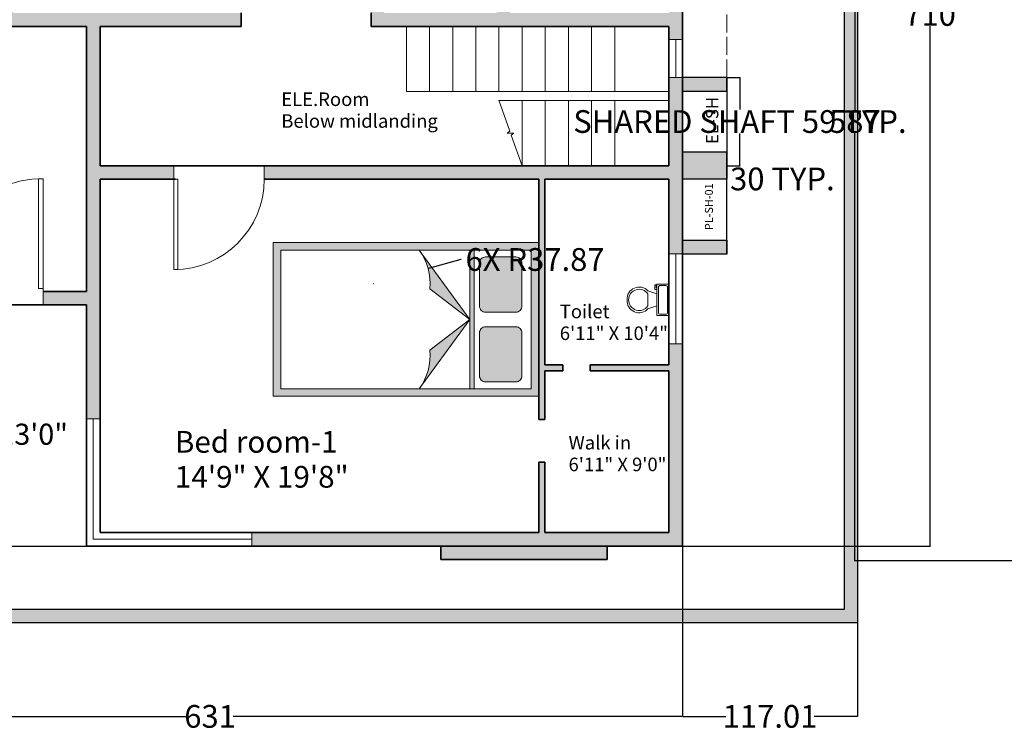
# Model space of a CAD drawing. Units: inches. Extents: x -828 to 1568, y -491 to 539.
# Tile 2 of 6: x -416 to 241, y -491 to -16. Entities that reach past the tile are written whole.
import ezdxf

# ---------------------------------------------------------------- set-up
doc = ezdxf.new("R2010")
doc.units = ezdxf.units.IN
doc.header["$MEASUREMENT"] = 0
doc.linetypes.add('ACAD_ISO02W100', pattern=[15, 12, -3])
for name, color, linetype, lineweight in [('A-ANNO-DIMS', 2, 'Continuous', 18), ('A-ANNO-TEXT', 7, 'Continuous', 18), ('A-AREA-IDEN', 7, 'Continuous', 18), ('A-DOOR', 3, 'Continuous', 18), ('A-FLOR-EDGE', 7, 'Continuous', 25), ('A-FLOR-FIXT', 9, 'Continuous', 18), ('A-FLOR-OVHD', 116, 'ACAD_ISO02W100', 13), ('A-FLOR-SHFT', 7, 'Continuous', 25), ('A-FLOR-STRS', 7, 'Continuous', 18), ('A-FURN', 8, 'Continuous', 18), ('A-FURN-PATT', 253, 'Continuous', 13), ('A-GLAZ', 4, 'Continuous', 18), ('A-WALL', 7, 'Continuous', 35), ('A-WALL-PATT', 8, 'Continuous', 13), ('L-SITE-PATT', 8, 'Continuous', 13), ('L-SITE-WALL', 7, 'Continuous', 30)]:
    doc.layers.add(name, color=color, linetype=linetype, lineweight=lineweight)
doc.styles.get("Standard").update_dxf_attribs({"font": 'arial.ttf'})
doc.dimstyles.get("Standard").update_dxf_attribs({"dimtxt": 15.18, "dimasz": 0.18, "dimexe": 0.18, "dimexo": 0.0625, "dimgap": 0.09, "dimtad": 0, "dimtih": 1, "dimtoh": 1, "dimdec": 0, "dimzin": 0, "dimdsep": 46, "dimlunit": 3, "dimtxsty": 'Standard', "dimcen": 0.09, "dimadec": 0, "dimazin": 0, "dimtfac": 1, "dimtdec": 0, "dimtofl": 0, "dimtmove": 0, "dimatfit": 3, "dimfxl": 1, "dimtolj": 1, "dimtzin": 0, "dimarcsym": 0})

# ---------------------------------------------------------------- blocks, each defined once
blk = doc.blocks.new('*U2')
for p, q in [((0, 0), (0, -6)), ((40, 0), (40, -6))]:
    blk.add_line(p, q)
blk.add_lwpolyline([(0, 0), (0, 40), (1.75, 40), (1.75, 0)], close=True)
blk.add_arc((0, 0), 40, 0, 90)
blk = doc.blocks.new('*U5')
for p, q in [((9.5, -6), (9.5, -2)), ((-10, -8.5), (-8, -8.5)), ((-10, -9.5), (-10, -8.5)), ((-7, -9.5), (-10, -9.5)), ((-8, -8.5), (-8, -8)), ((-7, -8), (-7, -9.5)), ((-4, -8), (-6, -14)), ((4, -8), (6, -14)), ((4, -14), (-4, -14))]:
    blk.add_line(p, q)
blk.add_lwpolyline([(10.5, -8), (10.5, 0), (-10.5, 0), (-10.5, -8)], close=True)
for points in [[(-9.5, -2), (-9.5, -6)], [(8.5, -1), (-8.5, -1)], [(-8.5, -7), (8.5, -7)]]:
    blk.add_lwpolyline(points)
for centre, radius, start, end in [((-8.625, -1.875), 0.8839, 81.8699, 188.1301), ((-8.625, -6.125), 0.8839, 171.869898, 278.1301), ((8.625, -1.875), 0.8839, 351.8699, 98.1301), ((8.625, -6.125), 0.8839, 261.8699, 8.1301), ((-0.4772, -19.9188), 8.0953, 133.01722, 273.38), ((0.0374, -19.8731), 7.127, 124.50543, 269.7), ((-0.0373, -19.8731), 7.127, 270.3, 55.4946), ((0.4773, -19.9188), 8.0953, 266.62, 46.9828)]:
    blk.add_arc(centre, radius, start, end)
blk = doc.blocks.new('SERVICE-SHAFT-59-SHARED-WALL')
for p, q in [((29.56, 58.98), (0, 58.98)), ((29.56, 49.77), (29.56, 58.98)), ((29.56, 58.98), (29.56, 0)), ((0, 49.77), (29.56, 49.77)), ((29.56, 9), (0, 9)), ((29.56, 0), (29.56, 9))]:
    blk.add_line(p, q)
blk = doc.blocks.new('BED-LINENS-DOUBLE')
h = blk.add_hatch(color=256)
h.dxf.hatch_style = 1
h.paths.add_polyline_path([(0, 92.62, -0.182673), (7.08, 66.8), (33.7, 46.31)])
h.paths.add_polyline_path([(33.7, 46.31), (7.08, 25.82, -0.182673), (0, 0)])
h = blk.add_hatch(color=256)
h.dxf.hatch_style = 1
h.paths.add_polyline_path([(36.7, 46.31), (33.7, 46.31), (33.7, 0), (36.7, 0)])
h.paths.add_polyline_path([(36.7, 92.62), (33.7, 92.62), (33.7, 46.31), (36.7, 46.31)])
h = blk.add_hatch(color=256)
h.dxf.hatch_style = 1
h.paths.add_polyline_path([(68.49, 84.07, 0.414214), (64.49, 88.07), (44.24, 88.07, 0.414214), (40.24, 84.07), (40.24, 55.21, 0.414214), (44.24, 51.21), (64.49, 51.21, 0.414214), (68.49, 55.21)])
h = blk.add_hatch(color=256)
h.dxf.hatch_style = 1
h.paths.add_polyline_path([(68.49, 37.42, 0.414214), (64.49, 41.42), (44.24, 41.42, 0.414214), (40.24, 37.42), (40.24, 8.55, 0.414214), (44.24, 4.55), (64.49, 4.55, 0.414214), (68.49, 8.55)])
for p, q in [((33.7, 46.31), (0, 92.62)), ((33.7, 0), (33.7, 92.62)), ((36.7, 0), (36.7, 92.62)), ((33.7, 46.31), (7.08, 66.8)), ((33.7, 46.31), (0, 0)), ((33.7, 46.31), (7.08, 25.82))]:
    blk.add_line(p, q)
for points in [[(64.49, 51.21), (44.24, 51.21, -0.414214), (40.24, 55.21), (40.24, 84.07, -0.414214), (44.24, 88.07), (64.49, 88.07, -0.414214), (68.49, 84.07), (68.49, 55.21, -0.414214)], [(64.49, 41.42), (44.24, 41.42, 0.414214), (40.24, 37.42), (40.24, 8.55, 0.414214), (44.24, 4.55), (64.49, 4.55, 0.414214), (68.49, 8.55), (68.49, 37.42, 0.414214)]]:
    blk.add_lwpolyline(points, format="xyb", close=True)
for centre, start, end in [((-30.62, 70.34), 354.63295, 36.04187), ((-30.62, 22.28), 323.95813, 5.36705)]:
    blk.add_arc(centre, 37.87, start, end)
blk = doc.blocks.new('*D23')
at = {"layer": 'A-ANNO-DIMS', "color": 0, "lineweight": -2, "transparency": 16777216}
for p, q in [((56.09, -54.44), (65.05, -54.44)), ((64.87, -54.62), (64.87, -75.99)), ((64.87, -113.24), (64.87, -91.87)), ((56.09, -113.42), (65.05, -113.42))]:
    blk.add_line(p, q, dxfattribs=at)
at = {"layer": 'A-ANNO-DIMS', "color": 0, "lineweight": 20, "transparency": 16777216}
for points in [[(64.84, -54.62), (64.9, -54.62), (64.87, -54.44)], [(64.84, -113.24), (64.9, -113.24), (64.87, -113.42)]]:
    blk.add_solid(points, dxfattribs=at)
at = {"layer": 'DEFPOINTS', "color": 0, "lineweight": 20, "transparency": 16777216}
for p in [(56.02, -54.44), (64.87, -54.44), (56.02, -113.42)]:
    blk.add_point(p, dxfattribs=at)
at = {"layer": 'A-ANNO-DIMS', "color": 0, "transparency": 16777216, "insert": (64.87, -83.93), "char_height": 15.18, "attachment_point": 5}
blk.add_mtext('\\A1;SHARED SHAFT 59 TYP.', dxfattribs=at)
blk = doc.blocks.new('*D24')
at = {"layer": 'A-ANNO-DIMS', "color": 0, "lineweight": -2, "transparency": 16777216}
for p, q in [((26.46, -113.48), (26.46, -122.44)), ((56.02, -113.48), (56.02, -122.44)), ((26.64, -122.26), (55.84, -122.26)), ((56.02, -122.26), (56.2, -122.26))]:
    blk.add_line(p, q, dxfattribs=at)
at = {"layer": 'A-ANNO-DIMS', "color": 0, "lineweight": 20, "transparency": 16777216}
for points in [[(26.64, -122.23), (26.64, -122.29), (26.46, -122.26)], [(55.84, -122.23), (55.84, -122.29), (56.02, -122.26)]]:
    blk.add_solid(points, dxfattribs=at)
at = {"layer": 'DEFPOINTS', "color": 0, "lineweight": 20, "transparency": 16777216}
for p in [(26.46, -113.42), (56.02, -113.42), (56.02, -122.26)]:
    blk.add_point(p, dxfattribs=at)
at = {"layer": 'A-ANNO-DIMS', "color": 0, "transparency": 16777216, "insert": (93.23, -122.26), "char_height": 15.18, "attachment_point": 5}
blk.add_mtext('\\A1;30 TYP.', dxfattribs=at)
blk = doc.blocks.new('*D33')
at = {"layer": 'A-ANNO-DIMS', "color": 0, "lineweight": -2, "transparency": 16777216}
for p, q in [((-604.54, -367.48), (-604.54, -481.38)), ((26.46, -367.48), (26.46, -481.38)), ((-604.36, -481.2), (-304.47, -481.2)), ((26.28, -481.2), (-273.6, -481.2))]:
    blk.add_line(p, q, dxfattribs=at)
at = {"layer": 'A-ANNO-DIMS', "color": 0, "lineweight": 20, "transparency": 16777216}
for points in [[(-604.36, -481.17), (-604.36, -481.23), (-604.54, -481.2)], [(26.28, -481.17), (26.28, -481.23), (26.46, -481.2)]]:
    blk.add_solid(points, dxfattribs=at)
at = {"layer": 'DEFPOINTS', "color": 0, "lineweight": 20, "transparency": 16777216}
for p in [(-604.54, -367.42), (26.46, -367.42), (26.46, -481.2)]:
    blk.add_point(p, dxfattribs=at)
at = {"layer": 'A-ANNO-DIMS', "color": 0, "transparency": 16777216, "insert": (-289.04, -481.2), "char_height": 15.18, "attachment_point": 5}
blk.add_mtext('\\A1;631', dxfattribs=at)
blk = doc.blocks.new('*D34')
at = {"layer": 'A-ANNO-DIMS', "color": 0, "lineweight": -2, "transparency": 16777216}
for p, q in [((26.52, 342.58), (192.05, 342.58)), ((191.87, 342.4), (191.87, -4.57)), ((191.87, -367.24), (191.87, -20.26)), ((26.52, -367.42), (192.05, -367.42))]:
    blk.add_line(p, q, dxfattribs=at)
at = {"layer": 'A-ANNO-DIMS', "color": 0, "lineweight": 20, "transparency": 16777216}
for points in [[(191.84, 342.4), (191.9, 342.4), (191.87, 342.58)], [(191.84, -367.24), (191.9, -367.24), (191.87, -367.42)]]:
    blk.add_solid(points, dxfattribs=at)
at = {"layer": 'DEFPOINTS', "color": 0, "lineweight": 20, "transparency": 16777216}
for p in [(26.46, 342.58), (191.87, 342.58), (26.46, -367.42)]:
    blk.add_point(p, dxfattribs=at)
at = {"layer": 'A-ANNO-DIMS', "color": 0, "transparency": 16777216, "insert": (191.87, -12.42), "char_height": 15.18, "attachment_point": 5}
blk.add_mtext('\\A1;710', dxfattribs=at)
blk = doc.blocks.new('*D35')
at = {"layer": 'A-ANNO-DIMS', "color": 0, "lineweight": -2, "transparency": 16777216}
for p, q in [((26.46, -367.48), (26.46, -481.38)), ((143.47, -418.8), (143.47, -481.38)), ((26.64, -481.2), (55.55, -481.2)), ((143.29, -481.2), (114.39, -481.2))]:
    blk.add_line(p, q, dxfattribs=at)
at = {"layer": 'A-ANNO-DIMS', "color": 0, "lineweight": 20, "transparency": 16777216}
for points in [[(26.64, -481.17), (26.64, -481.23), (26.46, -481.2)], [(143.29, -481.17), (143.29, -481.23), (143.47, -481.2)]]:
    blk.add_solid(points, dxfattribs=at)
at = {"layer": 'DEFPOINTS', "color": 0, "lineweight": 20, "transparency": 16777216}
for p in [(26.46, -367.42), (143.47, -418.73), (26.46, -481.2)]:
    blk.add_point(p, dxfattribs=at)
at = {"layer": 'A-ANNO-DIMS', "color": 0, "transparency": 16777216, "insert": (84.97, -481.2), "char_height": 15.18, "attachment_point": 5}
blk.add_mtext('\\A1;117.01', dxfattribs=at)
blk = doc.blocks.new('*D42')
at = {"layer": 'A-ANNO-DIMS', "color": 0, "lineweight": -2, "transparency": 16777216}
for p, q in [((347.86, 209.58), (141.48, 209.58)), ((141.66, 209.4), (141.66, -76.07)), ((141.66, -377.24), (141.66, -91.76)), ((279.86, -377.42), (141.48, -377.42))]:
    blk.add_line(p, q, dxfattribs=at)
at = {"layer": 'A-ANNO-DIMS', "color": 0, "lineweight": 20, "transparency": 16777216}
for points in [[(141.63, 209.4), (141.69, 209.4), (141.66, 209.58)], [(141.63, -377.24), (141.69, -377.24), (141.66, -377.42)]]:
    blk.add_solid(points, dxfattribs=at)
at = {"layer": 'DEFPOINTS', "color": 0, "lineweight": 20, "transparency": 16777216}
for p in [(141.66, 209.58), (347.92, 209.58), (279.92, -377.42)]:
    blk.add_point(p, dxfattribs=at)
at = {"layer": 'A-ANNO-DIMS', "color": 0, "transparency": 16777216, "insert": (141.66, -83.92), "char_height": 15.18, "attachment_point": 5}
blk.add_mtext('\\A1;587', dxfattribs=at)
blk = doc.blocks.new('*D55')
at = {"layer": 'A-ANNO-DIMS', "color": 0, "lineweight": -2, "transparency": 16777216}
for p, q in [((-121.48, -176.06), (-143.22, -182.02)), ((-121.3, -176.06), (-121.48, -176.06)), ((-180, -192.08), (-179.82, -192.08)), ((-179.91, -192.17), (-179.91, -191.99))]:
    blk.add_line(p, q, dxfattribs=at)
at = {"layer": 'A-ANNO-DIMS', "color": 0, "lineweight": 20, "transparency": 16777216}
blk.add_solid([(-143.22, -181.99), (-143.21, -182.05), (-143.39, -182.07)], dxfattribs=at)
at = {"layer": 'DEFPOINTS', "color": 0, "lineweight": 20, "transparency": 16777216}
for p in [(-143.39, -182.07), (-179.91, -192.08)]:
    blk.add_point(p, dxfattribs=at)
at = {"layer": 'A-ANNO-DIMS', "color": 0, "transparency": 16777216, "insert": (-71.98, -176.06), "char_height": 15.18, "attachment_point": 5}
blk.add_mtext('\\A1;6X R37.87', dxfattribs=at)

msp = doc.modelspace()

# ---------------------------------------------------------------- hatches: boundary and pattern name
at = {"layer": 'A-FURN-PATT'}
h = msp.add_hatch(color=256, dxfattribs=at)
h.dxf.hatch_style = 1
h.paths.add_polyline_path([(-69.5391, -164.8014), (-246.7968, -164.8014), (-246.7968, -267.4231), (-69.5391, -267.4231)])
h.paths.add_polyline_path([(-241.7968, -169.8014), (-74.5391, -169.8014), (-74.5391, -262.4231), (-241.7968, -262.4231)], flags=16)
at = {"layer": 'A-WALL-PATT'}
h = msp.add_hatch(color=256, dxfattribs=at)
h.dxf.hatch_style = 1
h.paths.add_polyline_path([(-473.7903, -197.4155), (-523.4337, -197.4155), (-523.4337, -206.4155), (-473.7903, -206.4155)])
h.paths.add_polyline_path([(-572.3651, -197.4155), (-595.5391, -197.4155), (-595.5391, -20.4155), (-520.2134, -20.4155), (-520.2134, -11.4155), (-604.5391, -11.4155), (-604.5391, -206.4155), (-572.3651, -206.4155)])
h.paths.add_polyline_path([(-604.5391, -170.4394), (-634.1027, -170.4394), (-634.1027, -179.4394), (-604.5391, -179.4394)])
h.paths.add_polyline_path([(-604.5391, -120.4631), (-634.1027, -120.4631), (-634.1027, -129.6673), (-604.5391, -129.6673)])
h.paths.add_polyline_path([(-268.3198, -11.4155), (-420.5391, -11.4155), (-420.5391, 9.0334), (-429.5391, 9.0334), (-429.5391, -11.4155), (-471.2821, -11.4155), (-471.2821, -20.4155), (-371.5391, -20.4155), (-371.5391, -197.4155), (-400.5108, -197.4155), (-400.5108, -206.4155), (-371.5391, -206.4155), (-371.5391, -282.4155), (-367.0391, -282.4155), (-362.5391, -282.4155), (-362.5391, -122.4155), (-313.1564, -122.4155), (-313.1564, -113.4155), (-362.5391, -113.4155), (-362.5391, -20.4155), (-268.3198, -20.4155)])
h.paths.add_polyline_path([(-313.539, 165.5845), (-375.5295, 165.5845), (-375.5295, 159.5845), (-313.539, 159.5845)])
h.paths.add_polyline_path([(-420.5391, 90.211), (-429.5391, 90.211), (-429.5391, 52.4437), (-420.5391, 52.4437)])
h.paths.add_polyline_path([(-420.5391, 211.3197), (-429.5391, 211.3197), (-429.5391, 134.8496), (-425.0391, 134.8496), (-420.5391, 134.8496), (-420.5391, 165.5845)])
h.paths.add_polyline_path([(-429.5391, 188.7113), (-438.5391, 188.7113), (-438.5391, 145.3797), (-429.5391, 145.3797)])
h.paths.add_polyline_path([(-517.0391, 342.5845), (-604.5391, 342.5845), (-604.5391, 333.5845), (-517.0391, 333.5845)])
h.paths.add_polyline_path([(-411.8784, 342.5845), (-429.5391, 342.5845), (-429.5391, 302.1645), (-420.5391, 302.1645), (-420.5391, 333.5845), (-411.8784, 333.5845)])
h.paths.add_polyline_path([(-311.8294, 372.1481), (-321.0336, 372.1481), (-321.0336, 342.5845), (-311.8294, 342.5845)])
h.paths.add_polyline_path([(-282.0163, 372.1481), (-291.2206, 372.1481), (-291.2206, 342.5845), (-282.0163, 342.5845)])
h.paths.add_polyline_path([(-230.7265, 342.5845), (-321.0336, 342.5845), (-321.0336, 333.5845), (-230.7265, 333.5845)])
h.paths.add_polyline_path([(-23.3113, 372.1481), (-32.5155, 372.1481), (-32.5155, 342.5845), (-23.3113, 342.5845)])
h.paths.add_polyline_path([(26.4609, 372.1481), (17.4609, 372.1481), (17.4609, 342.5845), (26.4609, 342.5845)])
h.paths.add_polyline_path([(56.6461, 259.1031), (26.4609, 259.1031), (26.4609, 248.5663), (56.6461, 248.5663)])
h.paths.add_polyline_path([(56.6461, 216.517), (26.4609, 216.517), (26.4609, 206.4193), (56.6461, 206.4193)])
h.paths.add_polyline_path([(56.0244, -54.4391), (26.4609, -54.4391), (26.4609, -63.6433), (56.0244, -63.6433)])
h.paths.add_polyline_path([(56.0244, -163.1876), (26.4609, -163.1876), (26.4609, -172.3918), (56.0244, -172.3918)])
h.paths.add_polyline_path([(56.0244, -113.4155), (56.0244, -104.4155), (26.4609, -104.4155), (26.4609, -122.4155), (56.0244, -122.4155)])
h.paths.add_polyline_path([(-23.844, -367.4155), (-134.8372, -367.4155), (-134.8372, -376.4155), (-23.844, -376.4155)])
h.paths.add_polyline_path([(26.4609, -54.4391), (21.9609, -54.4391), (17.4609, -54.4391), (17.4609, -113.4155), (-252.861, -113.4155), (-252.861, -122.4155), (-69.5391, -122.4155), (-69.5391, -282.9566), (-65.5391, -282.9566), (-65.5391, -250.4155), (-53.4738, -250.4155), (-53.4738, -246.4155), (-65.5391, -246.4155), (-65.5391, -122.4155), (17.4609, -122.4155), (17.4609, -172.3918), (26.4609, -172.3918), (26.4609, -163.1876)])
h.paths.add_polyline_path([(-172.5391, 156.5845), (-97.5391, 156.5845), (-97.5391, 62.5845), (-172.5391, 62.5845), (-172.5391, 98.9611, -0.05899862), (-178.0193, 98.3122), (-181.5391, 98.3122), (-181.5391, 33.9683), (-172.5391, 33.9683), (-172.5391, 53.5845), (-97.5391, 53.5845), (-97.5391, -11.4155), (-172.5391, -11.4155), (-172.5391, 9.9791), (-181.5391, 9.9791), (-181.5391, -11.4155), (-181.5391, -20.4155), (17.4609, -20.4155), (17.4609, -29.0707), (26.4609, -29.0707), (26.4609, 17.0407), (17.4609, 17.0407), (17.4609, -11.4155), (-88.5391, -11.4155), (-88.5391, 82.5845), (17.4609, 82.5845), (17.4609, 68.3133), (22.9411, 68.3133), (26.4609, 68.3133), (26.4609, 113.8123), (23.0131, 113.8123), (17.4609, 113.8123), (17.4609, 91.5845), (-88.5391, 91.5845), (-88.5391, 156.5845), (17.4609, 156.5845), (17.4609, 136.6113, -0.05979118), (23.0131, 137.2776), (26.4609, 137.2776), (26.4609, 259.1031), (21.9609, 259.1031), (17.4609, 259.1031), (17.4609, 237.5845), (-88.5391, 237.5845), (-88.5391, 249.5845), (-94.0193, 249.5845), (-97.5391, 249.5845), (-97.5391, 217.6678), (-94.0193, 217.6678), (-88.5391, 217.6678), (-88.5391, 230.5845), (17.4609, 230.5845), (17.4609, 165.5845), (-88.5391, 165.5845), (-88.5391, 194.8514, -0.05899862), (-94.0193, 194.2024), (-97.5391, 194.2024), (-97.5391, 165.5845), (-276.9691, 165.5845), (-276.9691, 156.5845), (-181.5391, 156.5845), (-181.5391, 121.7776), (-178.0193, 121.7776), (-172.5391, 121.7776)])
h.paths.add_polyline_path([(-88.5391, 333.5845), (17.4609, 333.5845), (17.4609, 313.1897), (26.4609, 313.1897), (26.4609, 342.5845), (-139.8817, 342.5845), (-139.8817, 333.5845), (-97.5391, 333.5845), (-97.5391, 273.0499), (-94.0193, 273.0499, -0.05899862), (-88.5391, 272.401)])
h.paths.add_polyline_path([(26.4609, -232.3042), (17.4609, -232.3042), (17.4609, -246.4155), (-35.2489, -246.4155), (-35.2489, -250.4155), (17.4609, -250.4155), (17.4609, -358.4155), (-65.5391, -358.4155), (-65.5391, -311.3725), (-69.5391, -311.3725), (-69.5391, -358.4155), (-261.1271, -358.4155), (-261.1271, -367.4155), (26.4609, -367.4155)])
at = {"layer": 'L-SITE-PATT'}
h = msp.add_hatch(color=256, dxfattribs=at)
h.dxf.hatch_style = 1
h.paths.add_polyline_path([(-695.1383, -418.734), (-695.1383, -409.734), (-744.5156, -409.734), (-744.5156, 440.0429), (134.4735, 440.0429), (134.4735, -409.734), (-428.0987, -409.734), (-428.0987, -418.734), (143.4735, -418.734), (143.4735, 449.0429), (-753.5156, 449.0429), (-753.5156, -418.734)])

# ---------------------------------------------------------------- linework, layer by layer
at = {"layer": 'A-FLOR-EDGE'}
msp.add_line((-604.5391, -367.4155), (-371.5391, -367.4155), dxfattribs=at)
at = {"layer": 'A-FLOR-OVHD'}
msp.add_line((56.0244, -54.4391), (56.6461, 206.4193), dxfattribs=at)
at = {"layer": 'A-FLOR-STRS'}
for p, q in [((-157.9223, -63.9155), (-157.9223, -20.4155)), ((-142.4606, -63.9155), (-142.4606, -20.4155)), ((-126.9989, -63.9155), (-126.9989, -20.4155)), ((-111.5372, -63.9155), (-111.5372, -20.4155)), ((-96.0756, -63.9155), (-96.0756, -20.4155)), ((-80.6139, -63.9155), (-80.6139, -20.4155)), ((-65.1522, -63.9155), (-65.1522, -20.4155)), ((-49.6905, -63.9155), (-49.6905, -20.4155)), ((-34.2288, -63.9155), (-34.2288, -20.4155)), ((-18.7671, -63.9155), (-18.7671, -20.4155)), ((17.4609, -63.9155), (-157.9223, -63.9155)), ((17.4609, -69.9155), (-96.0756, -69.9155)), ((-80.6139, -69.9155), (-80.6139, -113.4155)), ((-65.1522, -69.9155), (-65.1522, -113.4155)), ((-49.6905, -69.9155), (-49.6905, -113.4155)), ((-34.2288, -69.9155), (-34.2288, -113.4155)), ((-18.7671, -69.9155), (-18.7671, -113.4155))]:
    msp.add_line(p, q, dxfattribs=at)
msp.add_lwpolyline([(-96.1358, -69.7459), (-88.8471, -90.2521), (-90.5375, -91.6489), (-86.1519, -91.682), (-87.8423, -93.0788), (-80.5536, -113.5851)], dxfattribs=at)
at = {"layer": 'A-FURN'}
for points in [[(-69.5391, -267.4231), (-246.7968, -267.4231), (-246.7968, -164.8014), (-69.5391, -164.8014)], [(-74.5391, -262.4231), (-241.7968, -262.4231), (-241.7968, -169.8014), (-74.5391, -169.8014)]]:
    msp.add_lwpolyline(points, close=True, dxfattribs=at)
at = {"layer": 'A-GLAZ'}
for p, q in [((17.4609, -54.4391), (17.4609, -29.0707)), ((17.4609, -29.0707), (26.4609, -29.0707)), ((21.9609, -54.4391), (21.9609, -29.0707)), ((26.4609, -29.0707), (26.4609, -54.4391)), ((26.4609, -54.4391), (17.4609, -54.4391)), ((26.4609, -54.4391), (21.9609, -54.4391)), ((26.4609, -172.3918), (17.4609, -172.3918)), ((17.4609, -172.3918), (17.4609, -232.3042)), ((26.4609, -172.3918), (21.9609, -172.3918)), ((21.9609, -172.3918), (21.9609, -232.3042)), ((26.4609, -232.3042), (26.4609, -172.3918)), ((17.4609, -232.3042), (26.4609, -232.3042)), ((-371.5391, -282.4155), (-362.5391, -282.4155)), ((-371.5391, -367.4155), (-371.5391, -282.4155)), ((-371.5391, -282.4155), (-367.0391, -282.4155)), ((-367.0391, -282.4155), (-367.0391, -362.9155)), ((-362.5391, -282.4155), (-362.5391, -358.4155)), ((-362.5391, -358.4155), (-261.1271, -358.4155)), ((-261.1271, -358.4155), (-261.1271, -367.4155)), ((-261.1271, -367.4155), (-371.5391, -367.4155)), ((-261.1271, -362.9155), (-367.0391, -362.9155)), ((-367.0391, -367.4155), (-261.1271, -367.4155)), ((-261.1271, -367.4155), (-261.1271, -362.9155))]:
    msp.add_line(p, q, dxfattribs=at)
at = {"layer": 'A-WALL'}
for p, q in [((26.4609, 342.5845), (26.4609, -367.4155)), ((-268.3198, -11.4155), (-268.3198, -20.4155)), ((-181.5391, -11.4155), (-181.5391, -20.4155)), ((-595.5391, -20.4155), (-371.5391, -20.4155)), ((-595.5391, -20.4155), (-371.5391, -20.4155)), ((-371.5391, -20.4155), (-371.5391, -197.4155)), ((-362.5391, -20.4155), (-362.5391, -113.4155)), ((-362.5391, -20.4155), (-268.3198, -20.4155)), ((-88.5391, -20.4155), (-181.5391, -20.4155)), ((-181.5391, -20.4155), (17.4609, -20.4155)), ((-88.5391, -20.4155), (17.4609, -20.4155)), ((17.4609, -20.4155), (17.4609, -113.4155)), ((-362.5391, -113.4155), (17.4609, -113.4155)), ((-371.5391, -122.4155), (-371.5391, -197.4155)), ((-362.5391, -122.4155), (-312.1298, -122.4155)), ((-362.5391, -122.4155), (-362.5391, -358.4155)), ((-362.5391, -122.4155), (-362.5391, -206.4155)), ((-252.861, -122.4155), (-69.5391, -122.4155)), ((-69.5391, -122.4155), (-69.5391, -282.9566)), ((-65.5391, -122.4155), (-65.5391, -246.4155)), ((-65.5391, -122.4155), (17.4609, -122.4155)), ((-65.5391, -122.4155), (17.4609, -122.4155)), ((17.4609, -122.4155), (17.4609, -246.4155)), ((17.4609, -122.4155), (17.4609, -246.4155)), ((-400.5108, -197.4155), (-371.5391, -197.4155)), ((-604.5391, -206.4155), (-371.5391, -206.4155)), ((-371.5391, -206.4155), (-371.5391, -358.4155)), ((-65.5391, -246.4155), (-53.4738, -246.4155)), ((-53.4738, -246.4155), (-53.4738, -250.4155)), ((-35.2489, -250.4155), (-35.2489, -246.4155)), ((-35.2489, -246.4155), (17.4609, -246.4155)), ((-65.5391, -250.4155), (-53.4738, -250.4155)), ((-65.5391, -250.4155), (-65.5391, -282.9566)), ((-35.2489, -250.4155), (17.4609, -250.4155)), ((17.4609, -250.4155), (17.4609, -358.4155)), ((17.4609, -250.4155), (17.4609, -358.4155)), ((-65.5391, -282.9566), (-69.5391, -282.9566)), ((-69.5391, -311.3725), (-69.5391, -311.3725)), ((-69.5391, -311.3725), (-65.5391, -311.3725)), ((-69.5391, -311.3725), (-69.5391, -358.4155)), ((-65.5391, -311.3725), (-65.5391, -358.4155)), ((-371.5391, -358.4155), (-371.5391, -367.4155)), ((-362.5391, -358.4155), (-69.5391, -358.4155)), ((-65.5391, -358.4155), (17.4609, -358.4155)), ((-65.5391, -358.4155), (17.4609, -358.4155)), ((-371.5391, -367.4155), (26.4609, -367.4155)), ((-134.8372, -367.4155), (-134.8372, -376.4155)), ((-23.844, -376.4155), (-23.844, -367.4155)), ((-134.8372, -376.4155), (-23.844, -376.4155))]:
    msp.add_line(p, q, dxfattribs=at)
at = {"layer": 'L-SITE-WALL'}
for points in [[(-695.1383, -418.734), (-753.5156, -418.734), (-753.5156, 449.0429), (143.4735, 449.0429), (143.4735, -418.734), (-548.5793, -418.734)], [(-695.1383, -409.734), (-744.5156, -409.734), (-744.5156, 440.0429), (134.4735, 440.0429), (134.4735, -409.734), (-548.5793, -409.734)]]:
    msp.add_lwpolyline(points, dxfattribs=at)

# ---------------------------------------------------------------- block references
at = {"layer": 'A-DOOR', "xscale": -1.507384433454677, "yscale": 1.507384433454677, "zscale": 1.507384433454677, "rotation": 180}
msp.add_blockref('*U2', (-313.1564, -122.4598), dxfattribs=at)
at = {"layer": 'A-DOOR', "xscale": -1.831987710751254, "yscale": 1.831987710751254, "zscale": 1.831987710751254}
msp.add_blockref('*U2', (-400.5108, -195.4235), dxfattribs=at)
at = {"layer": 'A-FLOR-FIXT', "rotation": 270.0002079578468}
msp.add_blockref('*U5', (17.4608, -203.043), dxfattribs=at)
at = {"layer": 'A-FLOR-SHFT'}
msp.add_blockref('SERVICE-SHAFT-59-SHARED-WALL', (26.461, -113.415), dxfattribs=at)
at = {"layer": 'A-FLOR-SHFT', "extrusion": (0, 0, -1), "zscale": -1, "rotation": 180}
msp.add_blockref('SERVICE-SHAFT-59-SHARED-WALL', (-26.461, -113.4159), dxfattribs=at)
at = {"layer": 'A-FURN'}
msp.add_blockref('BED-LINENS-DOUBLE', (-149.29, -262.423), dxfattribs=at)

# ---------------------------------------------------------------- texts
at = {"layer": 'A-ANNO-TEXT'}
for s, height, p in [('EL-SH', 8.2278, (50.4427, -98.9505)), ('PL-SH-01', 5.31788, (46.8199, -156.4518))]:
    msp.add_text(s, height=height, rotation=90, dxfattribs=at).set_placement(p)
at = {"layer": 'A-AREA-IDEN'}
for s, height, p in [('ELE.Room', 9.04554, (-241.4828, -73.559)), ('Below midlanding', 9.045542, (-241.4828, -88.0899)), ('Toilet', 9.04554, (-55.4607, -215.316)), ('6\'11" X 10\'4"', 9.045542, (-55.4607, -229.8468)), ('18\'8" X 13\'0"', 14.099277, (-496.6166, -299.8197)), ('Bed room-1', 14.53185, (-312.5497, -305.122)), ('Walk in', 9.04554, (-49.6129, -302.9134)), ('6\'11" X 9\'0"', 9.045542, (-49.6129, -317.4442)), ('14\'9" X 19\'8"', 14.531855, (-312.5497, -328.4661))]:
    msp.add_text(s, height=height, dxfattribs=at).set_placement(p)

# ---------------------------------------------------------------- dimensions: what is measured, and where the dimension line sits
at = {"layer": 'A-ANNO-DIMS'}
for base, p1, p2, picture, middle in [((191.8735, 342.5845), (26.4609, -367.4155), (26.4609, 342.5845), '*D34', (191.8735, -12.4155)), ((141.6607, 209.5845), (279.9226, -377.4155), (347.9226, 209.5845), '*D42', (141.6607, -83.9155))]:
    dim = msp.add_linear_dim(base=base, p1=p1, p2=p2, angle=90, dimstyle='Standard', override={"dimdec": 0, "dimlfac": 1, "dimrnd": 0, "dimzin": 0, "dimdsep": 46, "dimlunit": 2}, dxfattribs=at)
    dim.commit()
    dim.dimension.update_dxf_attribs({"geometry": picture, "text_midpoint": middle})
dim = msp.add_linear_dim(base=(64.8709, -54.4391), p1=(56.0244, -113.4155), p2=(56.0244, -54.4391), angle=90, text='SHARED SHAFT <> TYP.', dimstyle='Standard', override={"dimdec": 0, "dimlfac": 1, "dimrnd": 0, "dimzin": 0, "dimdsep": 46, "dimlunit": 2}, dxfattribs=at)
dim.commit()
dim.dimension.update_dxf_attribs({"geometry": '*D23', "text_midpoint": (64.8709, -83.9273)})
dim = msp.add_linear_dim(base=(56.0244, -122.2619), p1=(26.4609, -113.4155), p2=(56.0244, -113.4155), text='<> TYP.', dimstyle='Standard', override={"dimdec": 0, "dimlfac": 1, "dimrnd": 0, "dimzin": 0, "dimdsep": 46, "dimlunit": 2}, dxfattribs=at)
dim.commit()
dim.dimension.update_dxf_attribs({"geometry": '*D24', "text_midpoint": (93.2349, -122.2619)})
dim = msp.add_radius_dim(center=(-179.9123, -192.084), mpoint=(-143.3897, -182.0669), text='6X <>', dimstyle='Standard', override={"dimdec": 2, "dimlfac": 1, "dimrnd": 0, "dimzin": 0, "dimdsep": 46, "dimlunit": 2}, dxfattribs=at)
dim.commit()
dim.dimension.update_dxf_attribs({"geometry": '*D55', "text_midpoint": (-71.9798, -176.0566), "dimtype": 164})
for p1, override, picture, middle in [((-604.5391, -367.4155), {"dimdec": 0, "dimlfac": 1, "dimrnd": 0, "dimzin": 0, "dimdsep": 46, "dimlunit": 2}, '*D33', (-289.0391, -481.1993)), ((143.4735, -418.734), {"dimdec": 2, "dimlfac": 1, "dimrnd": 0, "dimzin": 0, "dimdsep": 46, "dimlunit": 2}, '*D35', (84.9672, -481.1993))]:
    dim = msp.add_linear_dim(base=(26.4609, -481.1993), p1=p1, p2=(26.4609, -367.4155), dimstyle='Standard', override=override, dxfattribs=at)
    dim.commit()
    dim.dimension.update_dxf_attribs({"geometry": picture, "text_midpoint": middle})

doc.saveas('drawing.dxf')
